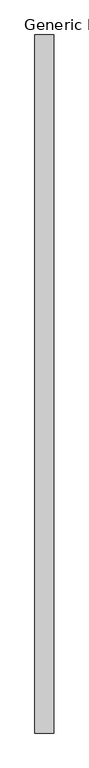
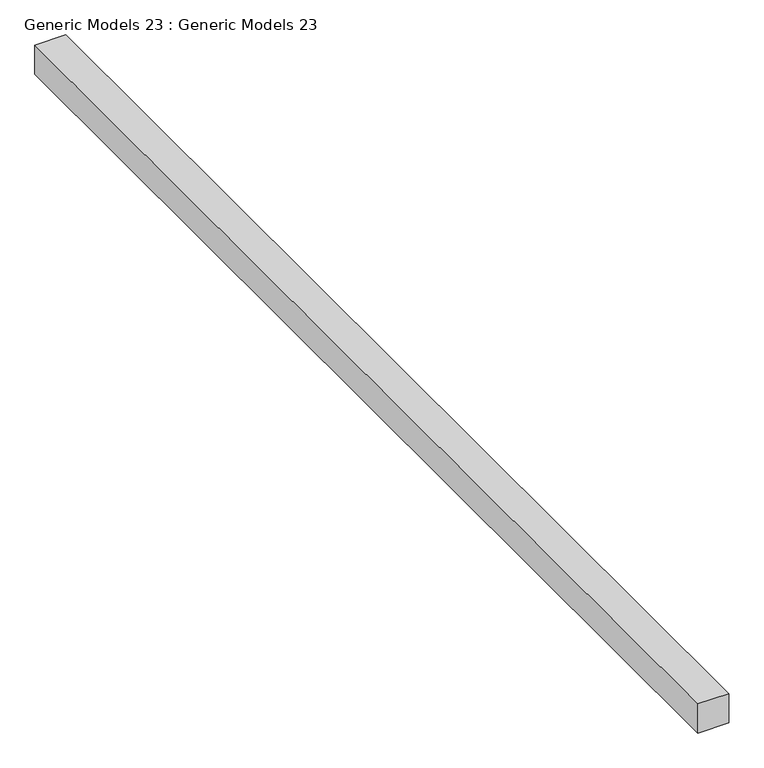
"""IFC4 building model written with IfcOpenShell, lengths in millimetres: proxy geometry, Generic Models 23 : Generic Models 23."""

from ifc_helpers import new_model, si_unit, frame, origin, place, context, project, spatial, polyline, outline, extrude, source, transform, mapped, element, save


def generic_models_23_generic_models_23_92ef9671(model_context):
    return source(origin(), model_context, "Body", "SweptSolid", [
        extrude(outline(polyline([(-15378.238074, -4372.9305222), (-15378.238074, 6941.8014639), (-15073.438074, 6941.8014639), (-15073.438074, -4372.9305222), (-15378.238074, -4372.9305222)])), frame((0.0, 0.0, 2743.2), z_axis=(0.0, 0.0, 1.0), x_axis=(1.0, 0.0, 0.0)), (0.0, 0.0, 1.0), 304.8),
    ])


if __name__ == "__main__":
    model = new_model("IFC4")
    model_context = context("Model", 3, world=origin())
    ifc_project = project(units=[si_unit("LENGTHUNIT", "METRE", prefix="MILLI")], contexts=[model_context])
    site = spatial("IfcSite", under=ifc_project)
    building = spatial("IfcBuilding", under=site)
    placement = place(None, origin())
    generic_models_23_generic_models_23_shape = generic_models_23_generic_models_23_92ef9671(model_context)
    element("IfcBuildingElementProxy", 1, Name="Generic Models 23 : Generic Models 23", ObjectType="Generic Models 23 : Generic Models 23", at=placement, inside=building, context=model_context, shape_type="MappedRepresentation", body=[
        mapped(generic_models_23_generic_models_23_shape, transform((0.0, 0.0, 0.0), x_axis=(1.0, 0.0, 0.0), y_axis=(0.0, 1.0, 0.0), z_axis=(0.0, 0.0, 1.0))),
    ])
    save(model, "model.ifc")
